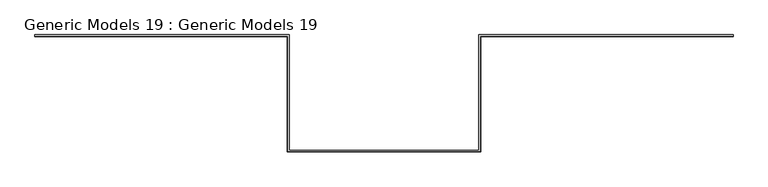
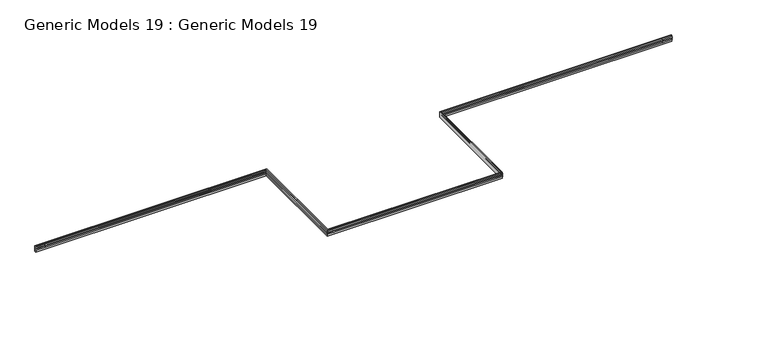
"""IFC4 building model written with IfcOpenShell, lengths in millimetres: proxy geometry, Generic Models 19 : Generic Models 19."""

from ifc_helpers import new_model, si_unit, frame, origin, place, context, project, spatial, circle_curve, ellipse_curve, source, transform, mapped, element, save
from ifc_brep_helpers import plane_surface, cylinder_surface, advanced_brep


def generic_models_19_generic_models_19_d22e943b(model_context):
    return source(origin(), model_context, "Body", "AdvancedBrep", [
        advanced_brep(
        [(6935.9174924, -5404.7542653, 6527.8), (6935.9174924, -5404.7542653, 6502.4), (6935.9174924, -5404.7542653, 6477.0), (6935.9174924, -5404.7542653, 6451.6), (6935.9174924, -5404.7542653, 6426.2), (6935.9174924, -5404.7542653, 6375.4), (6935.9174924, -5379.3542653, 6375.4), (6935.9174924, -5379.3542653, 6527.8), (1246.3174924, -5404.7542653, 6527.8), (1246.3174924, -5404.7542653, 6502.4), (6707.3174924, -5404.7542653, 6502.4), (6707.3174924, -5404.7542653, 6477.0), (1246.3174924, -5404.7542653, 6477.0), (1246.3174924, -5404.7542653, 6451.6), (6707.3174924, -5404.7542653, 6451.6), (6707.3174924, -5404.7542653, 6426.2), (1246.3174924, -5404.7542653, 6426.2), (1246.3174924, -5404.7542653, 6375.4), (1246.3174924, -8008.8292912, 6375.4), (-3071.6825076, -8008.8292912, 6375.4), (-3071.6825076, -5404.7542653, 6375.4), (-8761.2825076, -5404.7542653, 6375.4), (-8761.2825076, -5379.3542653, 6375.4), (-3046.2825076, -5379.3542653, 6375.4), (-3046.2825076, -7983.4292912, 6375.4), (1220.9174924, -7983.4292912, 6375.4), (1220.9174924, -5379.3542653, 6375.4), (1220.9174924, -5379.3542653, 6527.8), (1220.9174924, -7983.4292912, 6527.8), (-3046.2825076, -7983.4292912, 6527.8), (-3046.2825076, -5379.3542653, 6527.8), (-8761.2825076, -5379.3542653, 6527.8), (-8761.2825076, -5404.7542653, 6527.8), (-3071.6825076, -5404.7542653, 6527.8), (-3071.6825076, -8008.8292912, 6527.8), (1246.3174924, -8008.8292912, 6527.8), (1246.3174924, -8008.8292912, 6502.4), (1246.3174924, -7869.1292912, 6502.4), (1246.3174924, -7869.1292912, 6477.0), (1246.3174924, -8008.8292912, 6477.0), (1246.3174924, -8008.8292912, 6451.6), (1246.3174924, -7869.1292912, 6451.6), (1246.3174924, -7869.1292912, 6426.2), (1246.3174924, -8008.8292912, 6426.2), (-3071.6825076, -8008.8292912, 6502.4), (-2931.9825076, -8008.8292912, 6502.4), (-2931.9825076, -8008.8292912, 6477.0), (-3071.6825076, -8008.8292912, 6477.0), (-3071.6825076, -8008.8292912, 6451.6), (-2931.9825076, -8008.8292912, 6451.6), (-2931.9825076, -8008.8292912, 6426.2), (-3071.6825076, -8008.8292912, 6426.2), (-3071.6825076, -5404.7542653, 6502.4), (-3071.6825076, -5404.7542653, 6477.0), (-3071.6825076, -5404.7542653, 6451.6), (-3071.6825076, -5404.7542653, 6426.2), (-8761.2825076, -5404.7542653, 6502.4), (-8532.6825076, -5404.7542653, 6502.4), (-8532.6825076, -5404.7542653, 6477.0), (-8761.2825076, -5404.7542653, 6477.0), (-8761.2825076, -5404.7542653, 6451.6), (-8532.6825076, -5404.7542653, 6451.6), (-8532.6825076, -5404.7542653, 6426.2), (-8761.2825076, -5404.7542653, 6426.2)],
        [
            (0, 1),
            (1, 2, circle_curve(frame((6935.9174924, -5404.7542653, 6489.7), z_axis=(1.0, 0.0, 0.0), x_axis=(0.0, 1.0, 0.0)), 12.7)),
            (2, 3),
            (3, 4, circle_curve(frame((6935.9174924, -5404.7542653, 6438.9), z_axis=(1.0, 0.0, 0.0), x_axis=(0.0, 1.0, 0.0)), 12.7)),
            (4, 5),
            (5, 6),
            (6, 7),
            (7, 0),
            (0, 8),
            (8, 9),
            (9, 10),
            (10, 1),
            (10, 11, circle_curve(frame((6707.3174924, -5404.7542653, 6489.7), z_axis=(1.0, 0.0, 0.0), x_axis=(0.0, 1.0, 0.0)), 12.7)),
            (11, 2),
            (11, 12),
            (12, 13),
            (13, 14),
            (14, 3),
            (14, 15, circle_curve(frame((6707.3174924, -5404.7542653, 6438.9), z_axis=(1.0, 0.0, 0.0), x_axis=(0.0, 1.0, 0.0)), 12.7)),
            (15, 4),
            (15, 16),
            (16, 17),
            (17, 5),
            (17, 18),
            (18, 19),
            (19, 20),
            (20, 21),
            (21, 22),
            (22, 23),
            (23, 24),
            (24, 25),
            (25, 26),
            (26, 6),
            (26, 27),
            (27, 7),
            (27, 28),
            (28, 29),
            (29, 30),
            (30, 31),
            (31, 32),
            (32, 33),
            (33, 34),
            (34, 35),
            (35, 8),
            (9, 12, ellipse_curve(frame((1246.3174924, -5404.7542653, 6489.7), z_axis=(0.7071067811865492, 0.7071067811865457, 0.0), x_axis=(0.7071067811865458, -0.7071067811865491, 0.0)), 17.9605122, 12.7)),
            (13, 16, ellipse_curve(frame((1246.3174924, -5404.7542653, 6438.9), z_axis=(0.7071067811865492, 0.7071067811865457, 0.0), x_axis=(0.7071067811865458, -0.7071067811865491, 0.0)), 17.9605122, 12.7)),
            (35, 36),
            (36, 37),
            (37, 9),
            (37, 38, circle_curve(frame((1246.3174924, -7869.1292912, 6489.7), z_axis=(0.0, 1.0, 0.0), x_axis=(-1.0, 0.0, 0.0)), 12.7)),
            (38, 12),
            (38, 39),
            (39, 40),
            (40, 41),
            (41, 13),
            (41, 42, circle_curve(frame((1246.3174924, -7869.1292912, 6438.9), z_axis=(0.0, 1.0, 0.0), x_axis=(-1.0, 0.0, 0.0)), 12.7)),
            (42, 16),
            (42, 43),
            (43, 18),
            (25, 28),
            (36, 39, ellipse_curve(frame((1246.3174924, -8008.8292912, 6489.7), z_axis=(0.7071067811865505, 0.7071067811865446, 0.0), x_axis=(-0.7071067811865445, 0.7071067811865506, 0.0)), 17.9605122, 12.7)),
            (40, 43, ellipse_curve(frame((1246.3174924, -8008.8292912, 6438.9), z_axis=(0.7071067811865505, 0.7071067811865446, 0.0), x_axis=(-0.7071067811865445, 0.7071067811865506, 0.0)), 17.9605122, 12.7)),
            (34, 44),
            (44, 45),
            (45, 36),
            (45, 46, circle_curve(frame((-2931.9825076, -8008.8292912, 6489.7), z_axis=(1.0, 0.0, 0.0), x_axis=(0.0, 1.0, 0.0)), 12.7)),
            (46, 39),
            (46, 47),
            (47, 48),
            (48, 49),
            (49, 40),
            (49, 50, circle_curve(frame((-2931.9825076, -8008.8292912, 6438.9), z_axis=(1.0, 0.0, 0.0), x_axis=(0.0, 1.0, 0.0)), 12.7)),
            (50, 43),
            (50, 51),
            (51, 19),
            (24, 29),
            (44, 47, ellipse_curve(frame((-3071.6825076, -8008.8292912, 6489.7), z_axis=(0.7071067811865468, -0.7071067811865481, 0.0), x_axis=(0.7071067811865485, 0.7071067811865467, 0.0)), 17.9605122, 12.7)),
            (48, 51, ellipse_curve(frame((-3071.6825076, -8008.8292912, 6438.9), z_axis=(0.7071067811865468, -0.7071067811865481, 0.0), x_axis=(0.7071067811865485, 0.7071067811865467, 0.0)), 17.9605122, 12.7)),
            (33, 52),
            (52, 44),
            (52, 53, ellipse_curve(frame((-3071.6825076, -5404.7542653, 6489.7), z_axis=(0.7071067811865457, -0.7071067811865492, 0.0), x_axis=(-0.7071067811865491, -0.707106781186546, 0.0)), 17.9605122, 12.7)),
            (53, 47),
            (53, 54),
            (54, 48),
            (54, 55, ellipse_curve(frame((-3071.6825076, -5404.7542653, 6438.9), z_axis=(0.7071067811865457, -0.7071067811865492, 0.0), x_axis=(-0.7071067811865491, -0.707106781186546, 0.0)), 17.9605122, 12.7)),
            (55, 51),
            (55, 20),
            (23, 30),
            (32, 56),
            (56, 57),
            (57, 52),
            (57, 58, circle_curve(frame((-8532.6825076, -5404.7542653, 6489.7), z_axis=(1.0, 0.0, 0.0), x_axis=(0.0, 1.0, 0.0)), 12.7)),
            (58, 53),
            (58, 59),
            (59, 60),
            (60, 61),
            (61, 54),
            (61, 62, circle_curve(frame((-8532.6825076, -5404.7542653, 6438.9), z_axis=(1.0, 0.0, 0.0), x_axis=(0.0, 1.0, 0.0)), 12.7)),
            (62, 55),
            (62, 63),
            (63, 21),
            (22, 31),
            (63, 60, circle_curve(frame((-8761.2825076, -5404.7542653, 6438.9), z_axis=(-1.0, 0.0, 0.0), x_axis=(0.0, 1.0, 0.0)), 12.7)),
            (59, 56, circle_curve(frame((-8761.2825076, -5404.7542653, 6489.7), z_axis=(-1.0, 0.0, 0.0), x_axis=(0.0, 1.0, 0.0)), 12.7)),
        ],
        [
            plane_surface(frame((6935.9174924, -5379.3542653, 6527.8), z_axis=(1.0, 0.0, 0.0), x_axis=(0.0, 0.0, -1.0))),
            plane_surface(frame((6935.9174924, -5404.7542653, 6527.8), z_axis=(0.0, -1.0, 0.0), x_axis=(-1.0, 0.0, 0.0))),
            cylinder_surface(frame((6935.9174924, -5404.7542653, 6489.7), z_axis=(1.0, 0.0, 0.0), x_axis=(0.0, 1.0, 0.0)), 12.7),
            plane_surface(frame((6935.9174924, -5404.7542653, 6477.0), z_axis=(0.0, -1.0, 0.0), x_axis=(-1.0, 0.0, 0.0))),
            cylinder_surface(frame((6935.9174924, -5404.7542653, 6438.9), z_axis=(1.0, 0.0, 0.0), x_axis=(0.0, 1.0, 0.0)), 12.7),
            plane_surface(frame((6935.9174924, -5404.7542653, 6426.2), z_axis=(0.0, -1.0, 0.0), x_axis=(-1.0, 0.0, 0.0))),
            plane_surface(frame((6935.9174924, -5404.7542653, 6375.4), z_axis=(0.0, 0.0, -1.0), x_axis=(-1.0, 0.0, 0.0))),
            plane_surface(frame((6935.9174924, -5379.3542653, 6375.4), z_axis=(0.0, 1.0, 0.0), x_axis=(-1.0, 0.0, 0.0))),
            plane_surface(frame((6935.9174924, -5379.3542653, 6527.8), z_axis=(0.0, 0.0, 1.0), x_axis=(-1.0, 0.0, 0.0))),
            cylinder_surface(frame((6707.3174924, -5404.7542653, 6489.7), z_axis=(1.0, 0.0, 0.0), x_axis=(0.0, 1.0, 0.0)), 12.7),
            cylinder_surface(frame((6707.3174924, -5404.7542653, 6438.9), z_axis=(1.0, 0.0, 0.0), x_axis=(0.0, 1.0, 0.0)), 12.7),
            plane_surface(frame((1246.3174924, -5404.7542653, 6527.8), z_axis=(1.0, 0.0, 0.0), x_axis=(0.0, -1.0, 0.0))),
            cylinder_surface(frame((1246.3174924, -5379.3542653, 6489.7), z_axis=(0.0, 1.0, 0.0), x_axis=(-1.0, 0.0, 0.0)), 12.7),
            plane_surface(frame((1246.3174924, -5404.7542653, 6477.0), z_axis=(1.0, 0.0, 0.0), x_axis=(0.0, -1.0, 0.0))),
            cylinder_surface(frame((1246.3174924, -5379.3542653, 6438.9), z_axis=(0.0, 1.0, 0.0), x_axis=(-1.0, 0.0, 0.0)), 12.7),
            plane_surface(frame((1246.3174924, -5404.7542653, 6426.2), z_axis=(1.0, 0.0, 0.0), x_axis=(0.0, -1.0, 0.0))),
            plane_surface(frame((1220.9174924, -5379.3542653, 6375.4), z_axis=(-1.0, 0.0, 0.0), x_axis=(0.0, -1.0, 0.0))),
            cylinder_surface(frame((1246.3174924, -7869.1292912, 6489.7), z_axis=(0.0, 1.0, 0.0), x_axis=(-1.0, 0.0, 0.0)), 12.7),
            cylinder_surface(frame((1246.3174924, -7869.1292912, 6438.9), z_axis=(0.0, 1.0, 0.0), x_axis=(-1.0, 0.0, 0.0)), 12.7),
            plane_surface(frame((1246.3174924, -8008.8292912, 6527.8), z_axis=(0.0, -1.0, 0.0), x_axis=(-1.0, 0.0, 0.0))),
            cylinder_surface(frame((1220.9174924, -8008.8292912, 6489.7), z_axis=(1.0, 0.0, 0.0), x_axis=(0.0, 1.0, 0.0)), 12.7),
            plane_surface(frame((1246.3174924, -8008.8292912, 6477.0), z_axis=(0.0, -1.0, 0.0), x_axis=(-1.0, 0.0, 0.0))),
            cylinder_surface(frame((1220.9174924, -8008.8292912, 6438.9), z_axis=(1.0, 0.0, 0.0), x_axis=(0.0, 1.0, 0.0)), 12.7),
            plane_surface(frame((1246.3174924, -8008.8292912, 6426.2), z_axis=(0.0, -1.0, 0.0), x_axis=(-1.0, 0.0, 0.0))),
            plane_surface(frame((1220.9174924, -7983.4292912, 6375.4), z_axis=(0.0, 1.0, 0.0), x_axis=(-1.0, 0.0, 0.0))),
            cylinder_surface(frame((-2931.9825076, -8008.8292912, 6489.7), z_axis=(1.0, 0.0, 0.0), x_axis=(0.0, 1.0, 0.0)), 12.7),
            cylinder_surface(frame((-2931.9825076, -8008.8292912, 6438.9), z_axis=(1.0, 0.0, 0.0), x_axis=(0.0, 1.0, 0.0)), 12.7),
            plane_surface(frame((-3071.6825076, -8008.8292912, 6527.8), z_axis=(-1.0, 0.0, 0.0), x_axis=(0.0, 1.0, 0.0))),
            cylinder_surface(frame((-3071.6825076, -7983.4292912, 6489.7), z_axis=(0.0, -1.0, 0.0), x_axis=(1.0, 0.0, 0.0)), 12.7),
            plane_surface(frame((-3071.6825076, -8008.8292912, 6477.0), z_axis=(-1.0, 0.0, 0.0), x_axis=(0.0, 1.0, 0.0))),
            cylinder_surface(frame((-3071.6825076, -7983.4292912, 6438.9), z_axis=(0.0, -1.0, 0.0), x_axis=(1.0, 0.0, 0.0)), 12.7),
            plane_surface(frame((-3071.6825076, -8008.8292912, 6426.2), z_axis=(-1.0, 0.0, 0.0), x_axis=(0.0, 1.0, 0.0))),
            plane_surface(frame((-3046.2825076, -7983.4292912, 6375.4), z_axis=(1.0, 0.0, 0.0), x_axis=(0.0, 1.0, 0.0))),
            plane_surface(frame((-3071.6825076, -5404.7542653, 6527.8), z_axis=(0.0, -1.0, 0.0), x_axis=(-1.0, 0.0, 0.0))),
            cylinder_surface(frame((-3046.2825076, -5404.7542653, 6489.7), z_axis=(1.0, 0.0, 0.0), x_axis=(0.0, 1.0, 0.0)), 12.7),
            plane_surface(frame((-3071.6825076, -5404.7542653, 6477.0), z_axis=(0.0, -1.0, 0.0), x_axis=(-1.0, 0.0, 0.0))),
            cylinder_surface(frame((-3046.2825076, -5404.7542653, 6438.9), z_axis=(1.0, 0.0, 0.0), x_axis=(0.0, 1.0, 0.0)), 12.7),
            plane_surface(frame((-3071.6825076, -5404.7542653, 6426.2), z_axis=(0.0, -1.0, 0.0), x_axis=(-1.0, 0.0, 0.0))),
            plane_surface(frame((-3046.2825076, -5379.3542653, 6375.4), z_axis=(0.0, 1.0, 0.0), x_axis=(-1.0, 0.0, 0.0))),
            plane_surface(frame((-8761.2825076, -5379.3542653, 6527.8), z_axis=(-1.0, 0.0, 0.0), x_axis=(0.0, 0.0, -1.0))),
            cylinder_surface(frame((-8532.6825076, -5404.7542653, 6489.7), z_axis=(1.0, 0.0, 0.0), x_axis=(0.0, 1.0, 0.0)), 12.7),
            cylinder_surface(frame((-8532.6825076, -5404.7542653, 6438.9), z_axis=(1.0, 0.0, 0.0), x_axis=(0.0, 1.0, 0.0)), 12.7),
        ],
        [
            (0, [[1, 2, 3, 4, 5, 6, 7, 8]]),
            (1, [[-1, 9, 10, 11, 12]]),
            (2, [[-2, -12, 13, 14]]),
            (3, [[-3, -14, 15, 16, 17, 18]]),
            (4, [[-4, -18, 19, 20]]),
            (5, [[-5, -20, 21, 22, 23]]),
            (6, [[-6, -23, 24, 25, 26, 27, 28, 29, 30, 31, 32, 33]]),
            (7, [[-7, -33, 34, 35]]),
            (8, [[-9, -8, -35, 36, 37, 38, 39, 40, 41, 42, 43, 44]]),
            (9, [[-13, -11, 45, -15]]),
            (10, [[-19, -17, 46, -21]]),
            (11, [[-10, -44, 47, 48, 49]]),
            (12, [[-45, -49, 50, 51]]),
            (13, [[-16, -51, 52, 53, 54, 55]]),
            (14, [[-46, -55, 56, 57]]),
            (15, [[-24, -22, -57, 58, 59]]),
            (16, [[-36, -34, -32, 60]]),
            (17, [[-50, -48, 61, -52]]),
            (18, [[-56, -54, 62, -58]]),
            (19, [[-47, -43, 63, 64, 65]]),
            (20, [[-61, -65, 66, 67]]),
            (21, [[-53, -67, 68, 69, 70, 71]]),
            (22, [[-62, -71, 72, 73]]),
            (23, [[-25, -59, -73, 74, 75]]),
            (24, [[-37, -60, -31, 76]]),
            (25, [[-66, -64, 77, -68]]),
            (26, [[-72, -70, 78, -74]]),
            (27, [[-63, -42, 79, 80]]),
            (28, [[-77, -80, 81, 82]]),
            (29, [[-69, -82, 83, 84]]),
            (30, [[-78, -84, 85, 86]]),
            (31, [[-75, -86, 87, -26]]),
            (32, [[-76, -30, 88, -38]]),
            (33, [[-79, -41, 89, 90, 91]]),
            (34, [[-81, -91, 92, 93]]),
            (35, [[-83, -93, 94, 95, 96, 97]]),
            (36, [[-85, -97, 98, 99]]),
            (37, [[-27, -87, -99, 100, 101]]),
            (38, [[-39, -88, -29, 102]]),
            (39, [[-40, -102, -28, -101, 103, -95, 104, -89]]),
            (40, [[-92, -90, -104, -94]]),
            (41, [[-98, -96, -103, -100]]),
        ],
    ),
    ])


if __name__ == "__main__":
    model = new_model("IFC4")
    model_context = context("Model", 3, world=origin())
    ifc_project = project(units=[si_unit("LENGTHUNIT", "METRE", prefix="MILLI")], contexts=[model_context])
    site = spatial("IfcSite", under=ifc_project)
    building = spatial("IfcBuilding", under=site)
    placement = place(None, origin())
    generic_models_19_generic_models_19_shape = generic_models_19_generic_models_19_d22e943b(model_context)
    element("IfcBuildingElementProxy", 1, Name="Generic Models 19 : Generic Models 19", ObjectType="Generic Models 19 : Generic Models 19", at=placement, inside=building, context=model_context, shape_type="MappedRepresentation", body=[
        mapped(generic_models_19_generic_models_19_shape, transform((0.0, 0.0, 0.0), x_axis=(1.0, 0.0, 0.0), y_axis=(0.0, 1.0, 0.0), z_axis=(0.0, 0.0, 1.0))),
    ])
    save(model, "model.ifc")
